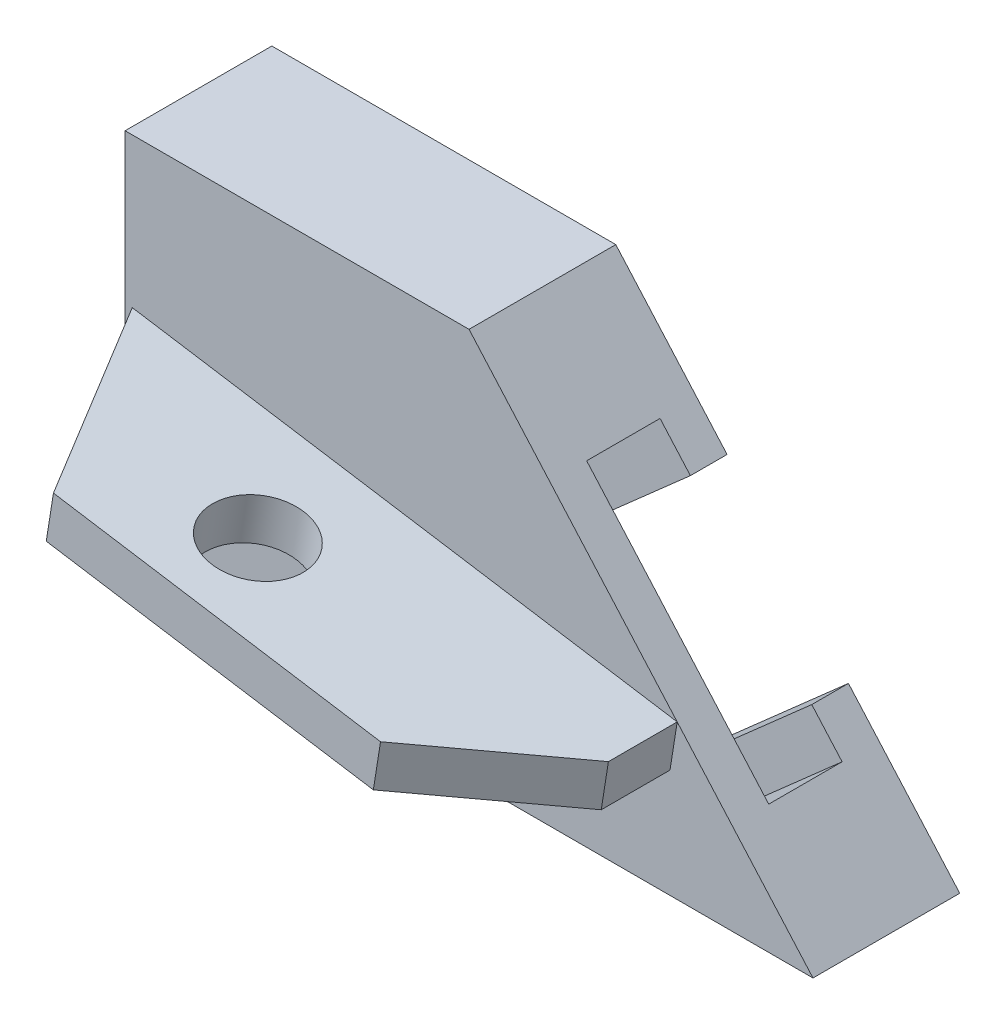
ISO-10303-21;
HEADER;
FILE_DESCRIPTION(('STEP AP214'),'2;1');
FILE_NAME('part.step','',(''),(''),'','','');
FILE_SCHEMA(('AUTOMOTIVE_DESIGN { 1 0 10303 214 1 1 1 1 }'));
ENDSEC;
DATA;
#1=APPLICATION_CONTEXT('core data for automotive mechanical design processes');
#2=APPLICATION_PROTOCOL_DEFINITION('international standard','automotive_design',2000,#1);
#3=PRODUCT_CONTEXT('',#1,'mechanical');
#4=PRODUCT('Part','Part','',(#3));
#5=PRODUCT_RELATED_PRODUCT_CATEGORY('part','',(#4));
#6=PRODUCT_DEFINITION_FORMATION('','',#4);
#7=PRODUCT_DEFINITION_CONTEXT('part definition',#1,'design');
#8=PRODUCT_DEFINITION('design','',#6,#7);
#9=PRODUCT_DEFINITION_SHAPE('','',#8);
#10=(LENGTH_UNIT() NAMED_UNIT(*) SI_UNIT(.MILLI.,.METRE.));
#11=(NAMED_UNIT(*) PLANE_ANGLE_UNIT() SI_UNIT($,.RADIAN.));
#12=(NAMED_UNIT(*) SI_UNIT($,.STERADIAN.) SOLID_ANGLE_UNIT());
#13=UNCERTAINTY_MEASURE_WITH_UNIT(LENGTH_MEASURE(1.E-05),#10,'distance_accuracy_value','');
#14=(GEOMETRIC_REPRESENTATION_CONTEXT(3) GLOBAL_UNCERTAINTY_ASSIGNED_CONTEXT((#13)) GLOBAL_UNIT_ASSIGNED_CONTEXT((#10,
#11,#12)) REPRESENTATION_CONTEXT('',''));
#15=CARTESIAN_POINT('',(0.,0.,0.));
#16=DIRECTION('',(0.,0.,1.));
#17=DIRECTION('',(1.,0.,0.));
#18=AXIS2_PLACEMENT_3D('',#15,#16,#17);
#19=CARTESIAN_POINT('',(0.,0.,0.));
#20=DIRECTION('',(0.,0.,-1.));
#21=DIRECTION('',(-1.,0.,0.));
#22=AXIS2_PLACEMENT_3D('',#19,#20,#21);
#23=PLANE('',#22);
#24=DIRECTION('',(-0.661621637086846,0.749837855365093,0.));
#25=VECTOR('',#24,1.);
#26=CARTESIAN_POINT('',(75.,85.,0.));
#27=LINE('',#26,#25);
#28=CARTESIAN_POINT('',(150.,0.,0.));
#29=VERTEX_POINT('',#28);
#30=CARTESIAN_POINT('',(120.391283670148,33.5565451738319,0.));
#31=VERTEX_POINT('',#30);
#32=EDGE_CURVE('E251',#29,#31,#27,.T.);
#33=ORIENTED_EDGE('',*,*,#32,.T.);
#34=DIRECTION('',(-0.156434465040224,-0.987688340595139,0.));
#35=VECTOR('',#34,1.);
#36=CARTESIAN_POINT('',(112.260327889279,-17.7802892033916,0.));
#37=LINE('',#36,#35);
#38=CARTESIAN_POINT('',(118.826939019746,23.6796617678805,0.));
#39=VERTEX_POINT('',#38);
#40=EDGE_CURVE('E179',#31,#39,#37,.T.);
#41=ORIENTED_EDGE('',*,*,#40,.T.);
#42=DIRECTION('',(0.987688340595139,-0.156434465040224,0.));
#43=VECTOR('',#42,1.);
#44=CARTESIAN_POINT('',(6.56661113046736,41.4599509712721,0.));
#45=LINE('',#44,#43);
#46=CARTESIAN_POINT('',(0.,42.5,0.));
#47=VERTEX_POINT('',#46);
#48=EDGE_CURVE('E184',#47,#39,#45,.T.);
#49=ORIENTED_EDGE('',*,*,#48,.F.);
#50=DIRECTION('',(0.,-1.,0.));
#51=VECTOR('',#50,1.);
#52=CARTESIAN_POINT('',(0.,0.,0.));
#53=LINE('',#52,#51);
#54=CARTESIAN_POINT('',(0.,0.,0.));
#55=VERTEX_POINT('',#54);
#56=EDGE_CURVE('E232',#47,#55,#53,.T.);
#57=ORIENTED_EDGE('',*,*,#56,.T.);
#58=DIRECTION('',(1.,0.,0.));
#59=VECTOR('',#58,1.);
#60=CARTESIAN_POINT('',(0.,0.,0.));
#61=LINE('',#60,#59);
#62=EDGE_CURVE('E246',#55,#29,#61,.T.);
#63=ORIENTED_EDGE('',*,*,#62,.T.);
#64=EDGE_LOOP('',(#33,#41,#49,#57,#63));
#65=FACE_BOUND('',#64,.T.);
#66=ADVANCED_FACE('F41',(#65),#23,.F.);
#67=CARTESIAN_POINT('',(0.,0.,-32.));
#68=DIRECTION('',(0.,0.,-1.));
#69=DIRECTION('',(-1.,0.,0.));
#70=AXIS2_PLACEMENT_3D('',#67,#68,#69);
#71=PLANE('',#70);
#72=DIRECTION('',(0.749837855365093,0.661621637086846,0.));
#73=VECTOR('',#72,1.);
#74=CARTESIAN_POINT('',(14.9290458574848,-16.9195853051495,-32.));
#75=LINE('',#74,#73);
#76=CARTESIAN_POINT('',(34.1045758699876,0.,-32.));
#77=VERTEX_POINT('',#76);
#78=CARTESIAN_POINT('',(99.2675672582631,57.4967571073019,-32.));
#79=VERTEX_POINT('',#78);
#80=EDGE_CURVE('E268',#77,#79,#75,.T.);
#81=ORIENTED_EDGE('',*,*,#80,.F.);
#82=DIRECTION('',(1.,0.,0.));
#83=VECTOR('',#82,1.);
#84=CARTESIAN_POINT('',(0.,0.,-32.));
#85=LINE('',#84,#83);
#86=CARTESIAN_POINT('',(0.,0.,-32.));
#87=VERTEX_POINT('',#86);
#88=EDGE_CURVE('E240',#87,#77,#85,.T.);
#89=ORIENTED_EDGE('',*,*,#88,.F.);
#90=DIRECTION('',(0.,-1.,0.));
#91=VECTOR('',#90,1.);
#92=CARTESIAN_POINT('',(0.,0.,-32.));
#93=LINE('',#92,#91);
#94=CARTESIAN_POINT('',(0.,85.,-32.));
#95=VERTEX_POINT('',#94);
#96=EDGE_CURVE('E234',#95,#87,#93,.T.);
#97=ORIENTED_EDGE('',*,*,#96,.F.);
#98=DIRECTION('',(-1.,0.,0.));
#99=VECTOR('',#98,1.);
#100=CARTESIAN_POINT('',(0.,85.,-32.));
#101=LINE('',#100,#99);
#102=CARTESIAN_POINT('',(75.,85.,-32.));
#103=VERTEX_POINT('',#102);
#104=EDGE_CURVE('E242',#103,#95,#101,.T.);
#105=ORIENTED_EDGE('',*,*,#104,.F.);
#106=DIRECTION('',(-0.661621637086846,0.749837855365093,0.));
#107=VECTOR('',#106,1.);
#108=CARTESIAN_POINT('',(75.,85.,-32.));
#109=LINE('',#108,#107);
#110=EDGE_CURVE('E238',#79,#103,#109,.T.);
#111=ORIENTED_EDGE('',*,*,#110,.F.);
#112=EDGE_LOOP('',(#81,#89,#97,#105,#111));
#113=FACE_BOUND('',#112,.T.);
#114=ADVANCED_FACE('F296',(#113),#71,.T.);
#115=CARTESIAN_POINT('',(0.,0.,-32.));
#116=DIRECTION('',(-1.,0.,0.));
#117=DIRECTION('',(0.,0.,1.));
#118=AXIS2_PLACEMENT_3D('',#115,#116,#117);
#119=PLANE('',#118);
#120=CARTESIAN_POINT('',(0.,85.,0.));
#121=VERTEX_POINT('',#120);
#122=EDGE_CURVE('E181',#121,#47,#53,.T.);
#123=ORIENTED_EDGE('',*,*,#122,.F.);
#124=DIRECTION('',(0.,0.,1.));
#125=VECTOR('',#124,1.);
#126=CARTESIAN_POINT('',(0.,85.,-32.));
#127=LINE('',#126,#125);
#128=EDGE_CURVE('E260',#95,#121,#127,.T.);
#129=ORIENTED_EDGE('',*,*,#128,.F.);
#130=ORIENTED_EDGE('',*,*,#96,.T.);
#131=DIRECTION('',(0.,0.,1.));
#132=VECTOR('',#131,1.);
#133=CARTESIAN_POINT('',(0.,0.,-32.));
#134=LINE('',#133,#132);
#135=EDGE_CURVE('E249',#87,#55,#134,.T.);
#136=ORIENTED_EDGE('',*,*,#135,.T.);
#137=ORIENTED_EDGE('',*,*,#56,.F.);
#138=EDGE_LOOP('',(#123,#129,#130,#136,#137));
#139=FACE_BOUND('',#138,.T.);
#140=ADVANCED_FACE('F43',(#139),#119,.T.);
#141=CARTESIAN_POINT('',(0.,85.,-32.));
#142=DIRECTION('',(0.,1.,0.));
#143=DIRECTION('',(0.,0.,1.));
#144=AXIS2_PLACEMENT_3D('',#141,#142,#143);
#145=PLANE('',#144);
#146=DIRECTION('',(-1.,0.,0.));
#147=VECTOR('',#146,1.);
#148=CARTESIAN_POINT('',(0.,85.,0.));
#149=LINE('',#148,#147);
#150=CARTESIAN_POINT('',(75.,85.,0.));
#151=VERTEX_POINT('',#150);
#152=EDGE_CURVE('E237',#151,#121,#149,.T.);
#153=ORIENTED_EDGE('',*,*,#152,.F.);
#154=DIRECTION('',(0.,0.,1.));
#155=VECTOR('',#154,1.);
#156=CARTESIAN_POINT('',(75.,85.,-32.));
#157=LINE('',#156,#155);
#158=EDGE_CURVE('E257',#103,#151,#157,.T.);
#159=ORIENTED_EDGE('',*,*,#158,.F.);
#160=ORIENTED_EDGE('',*,*,#104,.T.);
#161=ORIENTED_EDGE('',*,*,#128,.T.);
#162=EDGE_LOOP('',(#153,#159,#160,#161));
#163=FACE_BOUND('',#162,.T.);
#164=ADVANCED_FACE('F303',(#163),#145,.T.);
#165=CARTESIAN_POINT('',(75.,85.,-32.));
#166=DIRECTION('',(0.749837855365093,0.661621637086846,0.));
#167=DIRECTION('',(-0.661621637086846,0.749837855365093,0.));
#168=AXIS2_PLACEMENT_3D('',#165,#166,#167);
#169=PLANE('',#168);
#170=DIRECTION('',(0.,0.,1.));
#171=VECTOR('',#170,1.);
#172=CARTESIAN_POINT('',(99.2675672582631,57.4967571073019,-24.));
#173=LINE('',#172,#171);
#174=CARTESIAN_POINT('',(99.2675672582631,57.4967571073019,-24.));
#175=VERTEX_POINT('',#174);
#176=EDGE_CURVE('E215',#79,#175,#173,.T.);
#177=ORIENTED_EDGE('',*,*,#176,.F.);
#178=ORIENTED_EDGE('',*,*,#110,.T.);
#179=ORIENTED_EDGE('',*,*,#158,.T.);
#180=EDGE_CURVE('E252',#31,#151,#27,.T.);
#181=ORIENTED_EDGE('',*,*,#180,.F.);
#182=ORIENTED_EDGE('',*,*,#32,.F.);
#183=DIRECTION('',(0.,0.,1.));
#184=VECTOR('',#183,1.);
#185=CARTESIAN_POINT('',(150.,0.,-32.));
#186=LINE('',#185,#184);
#187=CARTESIAN_POINT('',(150.,0.,-32.));
#188=VERTEX_POINT('',#187);
#189=EDGE_CURVE('E263',#188,#29,#186,.T.);
#190=ORIENTED_EDGE('',*,*,#189,.F.);
#191=CARTESIAN_POINT('',(125.732432741737,27.5032428926981,-32.));
#192=VERTEX_POINT('',#191);
#193=EDGE_CURVE('E243',#188,#192,#109,.T.);
#194=ORIENTED_EDGE('',*,*,#193,.T.);
#195=DIRECTION('',(0.,0.,-1.));
#196=VECTOR('',#195,1.);
#197=CARTESIAN_POINT('',(125.732432741737,27.5032428926982,-24.));
#198=LINE('',#197,#196);
#199=CARTESIAN_POINT('',(125.732432741737,27.5032428926982,-24.));
#200=VERTEX_POINT('',#199);
#201=EDGE_CURVE('E209',#200,#192,#198,.T.);
#202=ORIENTED_EDGE('',*,*,#201,.F.);
#203=DIRECTION('',(-0.661621637086845,0.749837855365094,0.));
#204=VECTOR('',#203,1.);
#205=CARTESIAN_POINT('',(132.348649112605,20.0048643390473,-24.));
#206=LINE('',#205,#204);
#207=CARTESIAN_POINT('',(132.348649112605,20.0048643390473,-24.));
#208=VERTEX_POINT('',#207);
#209=EDGE_CURVE('E210',#208,#200,#206,.T.);
#210=ORIENTED_EDGE('',*,*,#209,.F.);
#211=DIRECTION('',(0.,0.,-1.));
#212=VECTOR('',#211,1.);
#213=CARTESIAN_POINT('',(132.348649112605,20.0048643390472,-8.00000000000001));
#214=LINE('',#213,#212);
#215=CARTESIAN_POINT('',(132.348649112605,20.0048643390472,-8.00000000000001));
#216=VERTEX_POINT('',#215);
#217=EDGE_CURVE('E204',#216,#208,#214,.T.);
#218=ORIENTED_EDGE('',*,*,#217,.F.);
#219=DIRECTION('',(0.661621637086846,-0.749837855365092,0.));
#220=VECTOR('',#219,1.);
#221=CARTESIAN_POINT('',(132.348649112605,20.0048643390472,-8.00000000000001));
#222=LINE('',#221,#220);
#223=CARTESIAN_POINT('',(92.6513508873946,64.9951356609528,-8.00000000000001));
#224=VERTEX_POINT('',#223);
#225=EDGE_CURVE('E203',#224,#216,#222,.T.);
#226=ORIENTED_EDGE('',*,*,#225,.F.);
#227=DIRECTION('',(0.,0.,1.));
#228=VECTOR('',#227,1.);
#229=CARTESIAN_POINT('',(92.6513508873946,64.9951356609528,-8.00000000000001));
#230=LINE('',#229,#228);
#231=CARTESIAN_POINT('',(92.6513508873946,64.9951356609528,-24.));
#232=VERTEX_POINT('',#231);
#233=EDGE_CURVE('E196',#232,#224,#230,.T.);
#234=ORIENTED_EDGE('',*,*,#233,.F.);
#235=DIRECTION('',(-0.661621637086847,0.749837855365092,0.));
#236=VECTOR('',#235,1.);
#237=CARTESIAN_POINT('',(99.2675672582631,57.4967571073019,-24.));
#238=LINE('',#237,#236);
#239=EDGE_CURVE('E193',#175,#232,#238,.T.);
#240=ORIENTED_EDGE('',*,*,#239,.F.);
#241=EDGE_LOOP('',(#177,#178,#179,#181,#182,#190,#194,#202,#210,#218,#226,#234,#240));
#242=FACE_BOUND('',#241,.T.);
#243=ADVANCED_FACE('F306',(#242),#169,.T.);
#244=CARTESIAN_POINT('',(0.,0.,-32.));
#245=DIRECTION('',(0.,-1.,0.));
#246=DIRECTION('',(0.,0.,-1.));
#247=AXIS2_PLACEMENT_3D('',#244,#245,#246);
#248=PLANE('',#247);
#249=DIRECTION('',(0.,0.,-1.));
#250=VECTOR('',#249,1.);
#251=CARTESIAN_POINT('',(34.1045758699876,0.,-32.));
#252=LINE('',#251,#250);
#253=CARTESIAN_POINT('',(34.1045758699876,0.,-24.));
#254=VERTEX_POINT('',#253);
#255=EDGE_CURVE('E227',#254,#77,#252,.T.);
#256=ORIENTED_EDGE('',*,*,#255,.F.);
#257=DIRECTION('',(1.,0.,0.));
#258=VECTOR('',#257,1.);
#259=CARTESIAN_POINT('',(0.,0.,-24.));
#260=LINE('',#259,#258);
#261=CARTESIAN_POINT('',(18.9901971383147,0.,-24.));
#262=VERTEX_POINT('',#261);
#263=EDGE_CURVE('E279',#262,#254,#260,.T.);
#264=ORIENTED_EDGE('',*,*,#263,.F.);
#265=DIRECTION('',(0.,0.,-1.));
#266=VECTOR('',#265,1.);
#267=CARTESIAN_POINT('',(18.9901971383148,0.,-32.));
#268=LINE('',#267,#266);
#269=CARTESIAN_POINT('',(18.9901971383147,0.,-8.00000000000001));
#270=VERTEX_POINT('',#269);
#271=EDGE_CURVE('E269',#270,#262,#268,.T.);
#272=ORIENTED_EDGE('',*,*,#271,.F.);
#273=DIRECTION('',(-1.,0.,0.));
#274=VECTOR('',#273,1.);
#275=CARTESIAN_POINT('',(0.,0.,-8.00000000000001));
#276=LINE('',#275,#274);
#277=CARTESIAN_POINT('',(109.676469528352,0.,-8.00000000000001));
#278=VERTEX_POINT('',#277);
#279=EDGE_CURVE('E275',#278,#270,#276,.T.);
#280=ORIENTED_EDGE('',*,*,#279,.F.);
#281=DIRECTION('',(0.,0.,1.));
#282=VECTOR('',#281,1.);
#283=CARTESIAN_POINT('',(109.676469528352,0.,-32.0000000000003));
#284=LINE('',#283,#282);
#285=CARTESIAN_POINT('',(109.676469528352,0.,-24.));
#286=VERTEX_POINT('',#285);
#287=EDGE_CURVE('E273',#286,#278,#284,.T.);
#288=ORIENTED_EDGE('',*,*,#287,.F.);
#289=DIRECTION('',(1.,0.,0.));
#290=VECTOR('',#289,1.);
#291=CARTESIAN_POINT('',(0.,0.,-24.));
#292=LINE('',#291,#290);
#293=CARTESIAN_POINT('',(94.562090796679,0.,-24.));
#294=VERTEX_POINT('',#293);
#295=EDGE_CURVE('E277',#294,#286,#292,.T.);
#296=ORIENTED_EDGE('',*,*,#295,.F.);
#297=DIRECTION('',(0.,0.,1.));
#298=VECTOR('',#297,1.);
#299=CARTESIAN_POINT('',(94.562090796679,0.,-32.));
#300=LINE('',#299,#298);
#301=CARTESIAN_POINT('',(94.562090796679,0.,-32.));
#302=VERTEX_POINT('',#301);
#303=EDGE_CURVE('E217',#302,#294,#300,.T.);
#304=ORIENTED_EDGE('',*,*,#303,.F.);
#305=EDGE_CURVE('E233',#302,#188,#85,.T.);
#306=ORIENTED_EDGE('',*,*,#305,.T.);
#307=ORIENTED_EDGE('',*,*,#189,.T.);
#308=ORIENTED_EDGE('',*,*,#62,.F.);
#309=ORIENTED_EDGE('',*,*,#135,.F.);
#310=ORIENTED_EDGE('',*,*,#88,.T.);
#311=EDGE_LOOP('',(#256,#264,#272,#280,#288,#296,#304,#306,#307,#308,#309,#310));
#312=FACE_BOUND('',#311,.T.);
#313=ADVANCED_FACE('F291',(#312),#248,.T.);
#314=DIRECTION('',(-0.749837855365093,-0.661621637086846,0.));
#315=VECTOR('',#314,1.);
#316=CARTESIAN_POINT('',(41.3939113409587,-46.9130995197532,-32.));
#317=LINE('',#316,#315);
#318=EDGE_CURVE('E259',#192,#302,#317,.T.);
#319=ORIENTED_EDGE('',*,*,#318,.F.);
#320=ORIENTED_EDGE('',*,*,#193,.F.);
#321=ORIENTED_EDGE('',*,*,#305,.F.);
#322=EDGE_LOOP('',(#319,#320,#321));
#323=FACE_BOUND('',#322,.T.);
#324=ADVANCED_FACE('F338',(#323),#71,.T.);
#325=ORIENTED_EDGE('',*,*,#122,.T.);
#326=DIRECTION('',(0.156434465040224,0.987688340595139,0.));
#327=VECTOR('',#326,1.);
#328=CARTESIAN_POINT('',(-6.56661113046736,1.0400490287279,0.));
#329=LINE('',#328,#327);
#330=CARTESIAN_POINT('',(1.56434465040224,52.3768834059514,0.));
#331=VERTEX_POINT('',#330);
#332=EDGE_CURVE('E165',#47,#331,#329,.T.);
#333=ORIENTED_EDGE('',*,*,#332,.T.);
#334=DIRECTION('',(0.987688340595139,-0.156434465040224,0.));
#335=VECTOR('',#334,1.);
#336=CARTESIAN_POINT('',(8.13095578086961,51.3368343772235,0.));
#337=LINE('',#336,#335);
#338=EDGE_CURVE('E166',#331,#31,#337,.T.);
#339=ORIENTED_EDGE('',*,*,#338,.T.);
#340=ORIENTED_EDGE('',*,*,#180,.T.);
#341=ORIENTED_EDGE('',*,*,#152,.T.);
#342=EDGE_LOOP('',(#325,#333,#339,#340,#341));
#343=FACE_BOUND('',#342,.T.);
#344=ADVANCED_FACE('F178',(#343),#23,.F.);
#345=CARTESIAN_POINT('',(-5.70973249284988,-35.1302720848566,-24.));
#346=DIRECTION('',(0.,0.,-1.));
#347=DIRECTION('',(-1.,0.,0.));
#348=AXIS2_PLACEMENT_3D('',#345,#346,#347);
#349=PLANE('',#348);
#350=ORIENTED_EDGE('',*,*,#263,.T.);
#351=DIRECTION('',(0.749837855365093,0.661621637086846,0.));
#352=VECTOR('',#351,1.);
#353=CARTESIAN_POINT('',(-5.70973249284988,-35.1302720848566,-24.));
#354=LINE('',#353,#352);
#355=EDGE_CURVE('E216',#254,#175,#354,.T.);
#356=ORIENTED_EDGE('',*,*,#355,.T.);
#357=ORIENTED_EDGE('',*,*,#239,.T.);
#358=DIRECTION('',(0.749837855365093,0.661621637086846,0.));
#359=VECTOR('',#358,1.);
#360=CARTESIAN_POINT('',(-12.3259488637184,-27.6318935312057,-24.));
#361=LINE('',#360,#359);
#362=EDGE_CURVE('E214',#262,#232,#361,.T.);
#363=ORIENTED_EDGE('',*,*,#362,.F.);
#364=EDGE_LOOP('',(#350,#356,#357,#363));
#365=FACE_BOUND('',#364,.T.);
#366=ADVANCED_FACE('F282',(#365),#349,.F.);
#367=CARTESIAN_POINT('',(-5.70973249284988,-35.1302720848566,-24.));
#368=DIRECTION('',(-0.661621637086846,0.749837855365093,0.));
#369=DIRECTION('',(-0.749837855365093,-0.661621637086846,0.));
#370=AXIS2_PLACEMENT_3D('',#367,#368,#369);
#371=PLANE('',#370);
#372=ORIENTED_EDGE('',*,*,#255,.T.);
#373=ORIENTED_EDGE('',*,*,#80,.T.);
#374=ORIENTED_EDGE('',*,*,#176,.T.);
#375=ORIENTED_EDGE('',*,*,#355,.F.);
#376=EDGE_LOOP('',(#372,#373,#374,#375));
#377=FACE_BOUND('',#376,.T.);
#378=ADVANCED_FACE('F286',(#377),#371,.F.);
#379=CARTESIAN_POINT('',(20.755132990624,-65.1237862994603,-24.));
#380=DIRECTION('',(0.661621637086846,-0.749837855365093,0.));
#381=DIRECTION('',(0.749837855365093,0.661621637086846,0.));
#382=AXIS2_PLACEMENT_3D('',#379,#380,#381);
#383=PLANE('',#382);
#384=ORIENTED_EDGE('',*,*,#303,.T.);
#385=DIRECTION('',(0.749837855365093,0.661621637086846,0.));
#386=VECTOR('',#385,1.);
#387=CARTESIAN_POINT('',(20.755132990624,-65.1237862994603,-24.));
#388=LINE('',#387,#386);
#389=EDGE_CURVE('E218',#294,#200,#388,.T.);
#390=ORIENTED_EDGE('',*,*,#389,.T.);
#391=ORIENTED_EDGE('',*,*,#201,.T.);
#392=ORIENTED_EDGE('',*,*,#318,.T.);
#393=EDGE_LOOP('',(#384,#390,#391,#392));
#394=FACE_BOUND('',#393,.T.);
#395=ADVANCED_FACE('F400',(#394),#383,.F.);
#396=CARTESIAN_POINT('',(27.3713493614924,-72.6221648531112,-24.));
#397=DIRECTION('',(0.,0.,-1.));
#398=DIRECTION('',(-1.,0.,0.));
#399=AXIS2_PLACEMENT_3D('',#396,#397,#398);
#400=PLANE('',#399);
#401=ORIENTED_EDGE('',*,*,#295,.T.);
#402=DIRECTION('',(0.749837855365093,0.661621637086846,0.));
#403=VECTOR('',#402,1.);
#404=CARTESIAN_POINT('',(27.3713493614924,-72.6221648531112,-24.));
#405=LINE('',#404,#403);
#406=EDGE_CURVE('E222',#286,#208,#405,.T.);
#407=ORIENTED_EDGE('',*,*,#406,.T.);
#408=ORIENTED_EDGE('',*,*,#209,.T.);
#409=ORIENTED_EDGE('',*,*,#389,.F.);
#410=EDGE_LOOP('',(#401,#407,#408,#409));
#411=FACE_BOUND('',#410,.T.);
#412=ADVANCED_FACE('F326',(#411),#400,.F.);
#413=CARTESIAN_POINT('',(27.3713493614924,-72.6221648531112,-8.00000000000001));
#414=DIRECTION('',(0.661621637086846,-0.749837855365093,0.));
#415=DIRECTION('',(0.749837855365093,0.661621637086846,0.));
#416=AXIS2_PLACEMENT_3D('',#413,#414,#415);
#417=PLANE('',#416);
#418=ORIENTED_EDGE('',*,*,#287,.T.);
#419=DIRECTION('',(0.749837855365093,0.661621637086846,0.));
#420=VECTOR('',#419,1.);
#421=CARTESIAN_POINT('',(27.3713493614924,-72.6221648531112,-8.00000000000001));
#422=LINE('',#421,#420);
#423=EDGE_CURVE('E224',#278,#216,#422,.T.);
#424=ORIENTED_EDGE('',*,*,#423,.T.);
#425=ORIENTED_EDGE('',*,*,#217,.T.);
#426=ORIENTED_EDGE('',*,*,#406,.F.);
#427=EDGE_LOOP('',(#418,#424,#425,#426));
#428=FACE_BOUND('',#427,.T.);
#429=ADVANCED_FACE('F325',(#428),#417,.F.);
#430=CARTESIAN_POINT('',(27.3713493614924,-72.6221648531112,-8.00000000000001));
#431=DIRECTION('',(0.,0.,1.));
#432=DIRECTION('',(1.,0.,0.));
#433=AXIS2_PLACEMENT_3D('',#430,#431,#432);
#434=PLANE('',#433);
#435=ORIENTED_EDGE('',*,*,#279,.T.);
#436=DIRECTION('',(0.749837855365093,0.661621637086846,0.));
#437=VECTOR('',#436,1.);
#438=CARTESIAN_POINT('',(-12.3259488637184,-27.6318935312057,-8.00000000000001));
#439=LINE('',#438,#437);
#440=EDGE_CURVE('E223',#270,#224,#439,.T.);
#441=ORIENTED_EDGE('',*,*,#440,.T.);
#442=ORIENTED_EDGE('',*,*,#225,.T.);
#443=ORIENTED_EDGE('',*,*,#423,.F.);
#444=EDGE_LOOP('',(#435,#441,#442,#443));
#445=FACE_BOUND('',#444,.T.);
#446=ADVANCED_FACE('F319',(#445),#434,.F.);
#447=CARTESIAN_POINT('',(-12.3259488637184,-27.6318935312057,-8.00000000000001));
#448=DIRECTION('',(-0.661621637086846,0.749837855365093,0.));
#449=DIRECTION('',(-0.749837855365093,-0.661621637086846,0.));
#450=AXIS2_PLACEMENT_3D('',#447,#448,#449);
#451=PLANE('',#450);
#452=ORIENTED_EDGE('',*,*,#271,.T.);
#453=ORIENTED_EDGE('',*,*,#362,.T.);
#454=ORIENTED_EDGE('',*,*,#233,.T.);
#455=ORIENTED_EDGE('',*,*,#440,.F.);
#456=EDGE_LOOP('',(#452,#453,#454,#455));
#457=FACE_BOUND('',#456,.T.);
#458=ADVANCED_FACE('F314',(#457),#451,.F.);
#459=CARTESIAN_POINT('',(112.260327889279,-17.7802892033916,40.));
#460=DIRECTION('',(0.987688340595139,-0.156434465040224,0.));
#461=DIRECTION('',(0.156434465040224,0.987688340595139,0.));
#462=AXIS2_PLACEMENT_3D('',#459,#460,#461);
#463=PLANE('',#462);
#464=DIRECTION('',(0.156434465040224,0.987688340595139,0.));
#465=VECTOR('',#464,1.);
#466=CARTESIAN_POINT('',(114.133905068539,-5.95098844997361,15.));
#467=LINE('',#466,#465);
#468=CARTESIAN_POINT('',(118.826939019746,23.6796617678805,15.));
#469=VERTEX_POINT('',#468);
#470=CARTESIAN_POINT('',(120.391283670148,33.5565451738319,15.));
#471=VERTEX_POINT('',#470);
#472=EDGE_CURVE('E413',#469,#471,#467,.T.);
#473=ORIENTED_EDGE('',*,*,#472,.F.);
#474=DIRECTION('',(0.,0.,-1.));
#475=VECTOR('',#474,1.);
#476=CARTESIAN_POINT('',(118.826939019746,23.6796617678805,40.));
#477=LINE('',#476,#475);
#478=EDGE_CURVE('E192',#469,#39,#477,.T.);
#479=ORIENTED_EDGE('',*,*,#478,.T.);
#480=ORIENTED_EDGE('',*,*,#40,.F.);
#481=DIRECTION('',(0.,0.,-1.));
#482=VECTOR('',#481,1.);
#483=CARTESIAN_POINT('',(120.391283670148,33.5565451738319,40.));
#484=LINE('',#483,#482);
#485=EDGE_CURVE('E171',#471,#31,#484,.T.);
#486=ORIENTED_EDGE('',*,*,#485,.F.);
#487=EDGE_LOOP('',(#473,#479,#480,#486));
#488=FACE_BOUND('',#487,.T.);
#489=ADVANCED_FACE('F393',(#488),#463,.T.);
#490=CARTESIAN_POINT('',(8.13095578086961,51.3368343772235,40.));
#491=DIRECTION('',(0.156434465040224,0.987688340595139,0.));
#492=DIRECTION('',(-0.987688340595139,0.156434465040224,0.));
#493=AXIS2_PLACEMENT_3D('',#490,#491,#492);
#494=PLANE('',#493);
#495=DIRECTION('',(-0.698401123333707,0.110615871041232,0.707106781186551));
#496=VECTOR('',#495,1.);
#497=CARTESIAN_POINT('',(120.391283670148,33.5565451738319,15.));
#498=LINE('',#497,#496);
#499=CARTESIAN_POINT('',(95.6990751552702,37.4674067998375,40.));
#500=VERTEX_POINT('',#499);
#501=EDGE_CURVE('E62',#471,#500,#498,.T.);
#502=ORIENTED_EDGE('',*,*,#501,.F.);
#503=ORIENTED_EDGE('',*,*,#485,.T.);
#504=ORIENTED_EDGE('',*,*,#338,.F.);
#505=DIRECTION('',(-0.493844170297564,0.0782172325201115,-0.866025403784442));
#506=VECTOR('',#505,1.);
#507=CARTESIAN_POINT('',(1.56434465040224,52.3768834059514,0.));
#508=LINE('',#507,#506);
#509=CARTESIAN_POINT('',(24.3740298231243,48.7641841858911,40.));
#510=VERTEX_POINT('',#509);
#511=EDGE_CURVE('E158',#510,#331,#508,.T.);
#512=ORIENTED_EDGE('',*,*,#511,.F.);
#513=DIRECTION('',(0.987688340595139,-0.156434465040224,0.));
#514=VECTOR('',#513,1.);
#515=CARTESIAN_POINT('',(8.13095578086961,51.3368343772235,40.));
#516=LINE('',#515,#514);
#517=EDGE_CURVE('E190',#510,#500,#516,.T.);
#518=ORIENTED_EDGE('',*,*,#517,.T.);
#519=EDGE_LOOP('',(#502,#503,#504,#512,#518));
#520=FACE_BOUND('',#519,.T.);
#521=CARTESIAN_POINT('',(50.9487616801592,44.5551601539402,22.));
#522=DIRECTION('',(0.156434465040224,0.987688340595139,0.));
#523=DIRECTION('',(-0.987688340595139,0.156434465040224,0.));
#524=AXIS2_PLACEMENT_3D('',#521,#522,#523);
#525=CIRCLE('',#524,10.);
#526=CARTESIAN_POINT('',(41.0718782742078,46.1195048043424,22.));
#527=VERTEX_POINT('',#526);
#528=EDGE_CURVE('E167',#527,#527,#525,.T.);
#529=ORIENTED_EDGE('',*,*,#528,.F.);
#530=EDGE_LOOP('',(#529));
#531=FACE_BOUND('',#530,.T.);
#532=ADVANCED_FACE('F168',(#520,#531),#494,.T.);
#533=CARTESIAN_POINT('',(6.56661113046736,41.4599509712721,40.));
#534=DIRECTION('',(0.156434465040224,0.987688340595139,0.));
#535=DIRECTION('',(-0.987688340595139,0.156434465040224,0.));
#536=AXIS2_PLACEMENT_3D('',#533,#534,#535);
#537=PLANE('',#536);
#538=CARTESIAN_POINT('',(49.3844170297569,34.6782767479888,22.));
#539=DIRECTION('',(0.156434465040224,0.987688340595139,0.));
#540=DIRECTION('',(-0.987688340595139,0.156434465040224,0.));
#541=AXIS2_PLACEMENT_3D('',#538,#539,#540);
#542=CIRCLE('',#541,10.);
#543=CARTESIAN_POINT('',(39.5075336238055,36.242621398391,22.));
#544=VERTEX_POINT('',#543);
#545=EDGE_CURVE('E44',#544,#544,#542,.T.);
#546=ORIENTED_EDGE('',*,*,#545,.T.);
#547=EDGE_LOOP('',(#546));
#548=FACE_BOUND('',#547,.T.);
#549=ORIENTED_EDGE('',*,*,#478,.F.);
#550=DIRECTION('',(-0.698401123333707,0.110615871041232,0.707106781186551));
#551=VECTOR('',#550,1.);
#552=CARTESIAN_POINT('',(50.3506708176681,34.525237182579,84.3298334987106));
#553=LINE('',#552,#551);
#554=CARTESIAN_POINT('',(94.1347305048679,27.5905233938861,40.));
#555=VERTEX_POINT('',#554);
#556=EDGE_CURVE('E350',#469,#555,#553,.T.);
#557=ORIENTED_EDGE('',*,*,#556,.T.);
#558=DIRECTION('',(0.987688340595139,-0.156434465040224,0.));
#559=VECTOR('',#558,1.);
#560=CARTESIAN_POINT('',(6.56661113046736,41.4599509712721,40.));
#561=LINE('',#560,#559);
#562=CARTESIAN_POINT('',(22.809685172722,38.8873007799397,40.));
#563=VERTEX_POINT('',#562);
#564=EDGE_CURVE('E195',#563,#555,#561,.T.);
#565=ORIENTED_EDGE('',*,*,#564,.F.);
#566=DIRECTION('',(-0.493844170297564,0.0782172325201113,-0.866025403784441));
#567=VECTOR('',#566,1.);
#568=CARTESIAN_POINT('',(18.7489166621584,39.5304633277728,32.8788696909858));
#569=LINE('',#568,#567);
#570=EDGE_CURVE('E60',#563,#47,#569,.T.);
#571=ORIENTED_EDGE('',*,*,#570,.T.);
#572=ORIENTED_EDGE('',*,*,#48,.T.);
#573=EDGE_LOOP('',(#549,#557,#565,#571,#572));
#574=FACE_BOUND('',#573,.T.);
#575=ADVANCED_FACE('F345',(#548,#574),#537,.F.);
#576=CARTESIAN_POINT('',(0.,0.,40.));
#577=DIRECTION('',(0.,0.,1.));
#578=DIRECTION('',(1.,0.,0.));
#579=AXIS2_PLACEMENT_3D('',#576,#577,#578);
#580=PLANE('',#579);
#581=DIRECTION('',(-0.156434465040224,-0.987688340595139,0.));
#582=VECTOR('',#581,1.);
#583=CARTESIAN_POINT('',(87.5681193744005,-13.869427577386,40.));
#584=LINE('',#583,#582);
#585=EDGE_CURVE('E11',#500,#555,#584,.T.);
#586=ORIENTED_EDGE('',*,*,#585,.F.);
#587=ORIENTED_EDGE('',*,*,#517,.F.);
#588=DIRECTION('',(0.156434465040224,0.987688340595139,0.));
#589=VECTOR('',#588,1.);
#590=CARTESIAN_POINT('',(16.2430740422547,-2.5726501913324,40.));
#591=LINE('',#590,#589);
#592=EDGE_CURVE('E49',#563,#510,#591,.T.);
#593=ORIENTED_EDGE('',*,*,#592,.F.);
#594=ORIENTED_EDGE('',*,*,#564,.T.);
#595=EDGE_LOOP('',(#586,#587,#593,#594));
#596=FACE_BOUND('',#595,.T.);
#597=ADVANCED_FACE('F406',(#596),#580,.T.);
#598=CARTESIAN_POINT('',(-4.69303395120673,12.8693497821459,0.));
#599=DIRECTION('',(0.85536319397709,-0.135476220752263,-0.499999999999995));
#600=DIRECTION('',(-0.504652595083946,0.,-0.86332251115967));
#601=AXIS2_PLACEMENT_3D('',#598,#599,#600);
#602=PLANE('',#601);
#603=ORIENTED_EDGE('',*,*,#592,.T.);
#604=ORIENTED_EDGE('',*,*,#511,.T.);
#605=ORIENTED_EDGE('',*,*,#332,.F.);
#606=ORIENTED_EDGE('',*,*,#570,.F.);
#607=EDGE_LOOP('',(#603,#604,#605,#606));
#608=FACE_BOUND('',#607,.T.);
#609=ADVANCED_FACE('F159',(#608),#602,.F.);
#610=CARTESIAN_POINT('',(114.133905068539,-5.95098844997361,15.));
#611=DIRECTION('',(-0.698401123333715,0.110615871041233,-0.707106781186544));
#612=DIRECTION('',(-0.711472923612858,0.,0.702713511301563));
#613=AXIS2_PLACEMENT_3D('',#610,#611,#612);
#614=PLANE('',#613);
#615=ORIENTED_EDGE('',*,*,#472,.T.);
#616=ORIENTED_EDGE('',*,*,#501,.T.);
#617=ORIENTED_EDGE('',*,*,#585,.T.);
#618=ORIENTED_EDGE('',*,*,#556,.F.);
#619=EDGE_LOOP('',(#615,#616,#617,#618));
#620=FACE_BOUND('',#619,.T.);
#621=ADVANCED_FACE('F363',(#620),#614,.F.);
#622=CARTESIAN_POINT('',(44.6913830785502,5.04762653013465,22.));
#623=DIRECTION('',(0.156434465040224,0.987688340595139,0.));
#624=DIRECTION('',(-0.987688340595139,0.156434465040224,0.));
#625=AXIS2_PLACEMENT_3D('',#622,#623,#624);
#626=CYLINDRICAL_SURFACE('',#625,10.);
#627=ORIENTED_EDGE('',*,*,#528,.T.);
#628=EDGE_LOOP('',(#627));
#629=FACE_BOUND('',#628,.T.);
#630=ORIENTED_EDGE('',*,*,#545,.F.);
#631=EDGE_LOOP('',(#630));
#632=FACE_BOUND('',#631,.T.);
#633=ADVANCED_FACE('F356',(#629,#632),#626,.F.);
#634=CLOSED_SHELL('',(#66,#114,#140,#164,#243,#313,#324,#344,#366,#378,#395,#412,#429,#446,#458,
#489,#532,#575,#597,#609,#621,#633));
#635=MANIFOLD_SOLID_BREP('B2',#634);
#636=ADVANCED_BREP_SHAPE_REPRESENTATION('',(#18,#635),#14);
#637=SHAPE_DEFINITION_REPRESENTATION(#9,#636);
ENDSEC;
END-ISO-10303-21;
